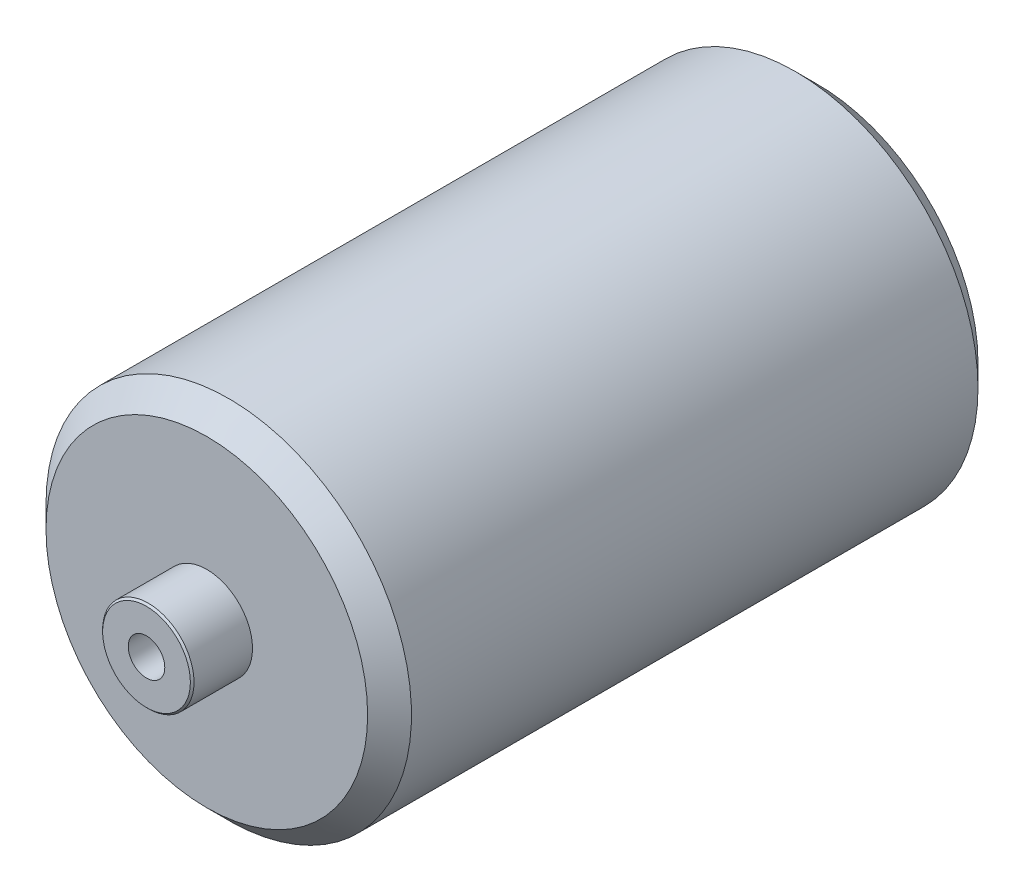
from build123d import *

# Parameters (mm, degrees)
BODY_PROFILE_100_R              = 50
MAIN_BODY_100X167_DEPTH         = 167
SPIGOT_1_PROFILE_25_R           = 12.5
END_SPIGOT_1_25X16_5_DEPTH      = 16.5
END_START                       = 16.5
SPIGOT_2_PROFILE_25_R           = 12.5
END_SPIGOT_2_25X16_5_DEPTH      = 16.5
SPIGOT_2_DOWEL_HOLE_10X59_D     = 10
SPIGOT_2_DOWEL_HOLE_10X59_DEPTH = 59
SPIGOT_2_DOWEL_HOLE_10X59_TIP   = 3.004303095
SPIGOT_1_DOWEL_HOLE_10X59_D     = 10
SPIGOT_1_DOWEL_HOLE_10X59_DEPTH = 59
SPIGOT_1_DOWEL_HOLE_10X59_TIP   = 3.004303095
SPIGOT_EDGE_CHAMFER_0_5_SIZE    = 0.5
BODY_EDGE_CHAMFER_6_SIZE        = 6


with BuildPart() as part:
    # Body Profile Ø100 → Main Body Ø100x167 (new body)
    with BuildSketch(Plane.XY):
        with Locations(Location((0, 0, 0), (0, 0, 180))):
            Circle(BODY_PROFILE_100_R)
    extrude(amount=MAIN_BODY_100X167_DEPTH)

    # Spigot 1 Profile Ø25 → End Spigot 1 Ø25x16.5 (add)
    with BuildSketch(Plane.XY.offset(167)):
        Circle(SPIGOT_1_PROFILE_25_R)
    extrude(amount=END_SPIGOT_1_25X16_5_DEPTH)

    # Spigot 2 Profile Ø25 → End Spigot 2 Ø25x16.5 (add)
    with BuildSketch(Plane(origin=(0, 0, 0), x_dir=(-1, 0, 0), z_dir=(0, 0, -1)).offset(END_START)):
        with Locations(Location((0, 0, 0), (0, 0, 180))):
            Circle(SPIGOT_2_PROFILE_25_R)
    extrude(amount=-END_SPIGOT_2_25X16_5_DEPTH)

    # Spigot 2 Dowel Hole Ø10x59
    with Locations(Plane(origin=(0, 0, -16.5), x_dir=(-1, 0, 0), z_dir=(0, 0, -1))):
        with Locations((0, 0)):
            Hole(SPIGOT_2_DOWEL_HOLE_10X59_D / 2, depth=SPIGOT_2_DOWEL_HOLE_10X59_DEPTH)
            with Locations((0, 0, -(SPIGOT_2_DOWEL_HOLE_10X59_DEPTH + SPIGOT_2_DOWEL_HOLE_10X59_TIP / 2))):  # 118° drill point
                Cone(0, SPIGOT_2_DOWEL_HOLE_10X59_D / 2, SPIGOT_2_DOWEL_HOLE_10X59_TIP, mode=Mode.SUBTRACT)

    # Spigot 1 Dowel Hole Ø10x59
    with Locations(Plane.XY.offset(183.5)):
        with Locations((0, 0)):
            Hole(SPIGOT_1_DOWEL_HOLE_10X59_D / 2, depth=SPIGOT_1_DOWEL_HOLE_10X59_DEPTH)
            with Locations((0, 0, -(SPIGOT_1_DOWEL_HOLE_10X59_DEPTH + SPIGOT_1_DOWEL_HOLE_10X59_TIP / 2))):  # 118° drill point
                Cone(0, SPIGOT_1_DOWEL_HOLE_10X59_D / 2, SPIGOT_1_DOWEL_HOLE_10X59_TIP, mode=Mode.SUBTRACT)

    # Spigot Edge Chamfer 0.5
    spigot_edge_chamfer_0_5_edges = [part.edges().sort_by_distance(p)[0] for p in [
        (-12.5, 0, -16.5),
        (-12.5, 0, 183.5),
    ]]
    chamfer(spigot_edge_chamfer_0_5_edges, length=SPIGOT_EDGE_CHAMFER_0_5_SIZE)

    # Body Edge Chamfer 6
    body_edge_chamfer_6_edges = [part.edges().sort_by_distance(p)[0] for p in [
        (50, 0, 0),
        (50, 0, 167),
    ]]
    chamfer(body_edge_chamfer_6_edges, length=BODY_EDGE_CHAMFER_6_SIZE)


solid = part.part
